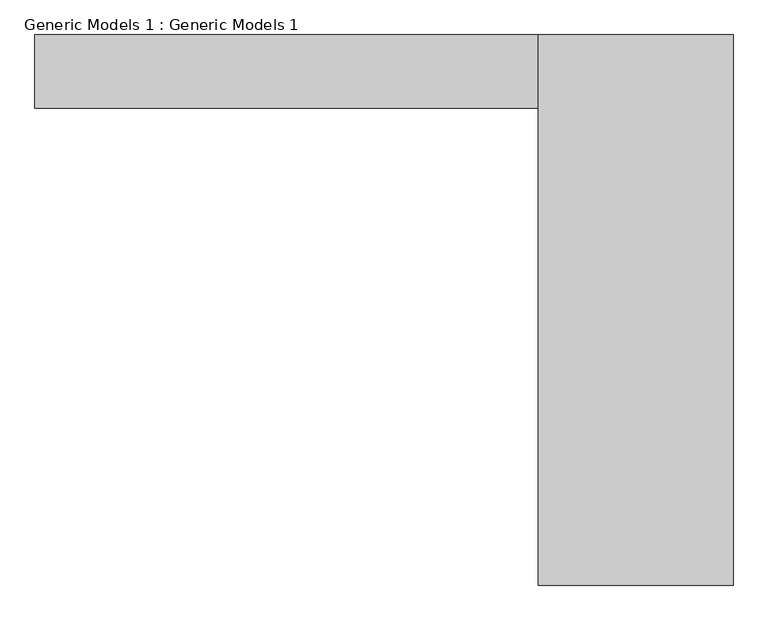
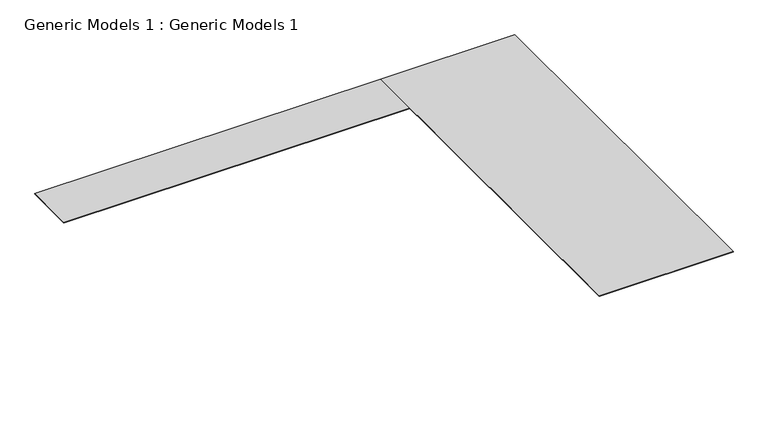
"""IFC4 building model written with IfcOpenShell, lengths in millimetres: proxy geometry, Generic Models 1 : Generic Models 1."""

from ifc_helpers import new_model, si_unit, origin, origin_with_axes, place, context, project, spatial, polyline, outline, extrude, source, transform, mapped, element, save


def generic_models_1_generic_models_1_28a2cc20(model_context):
    return source(origin(), model_context, "Body", "SweptSolid", [
        extrude(outline(polyline([(21968.4663282, 19178.0873915), (-9452.0005661, 19178.0873915), (-9452.0005661, 23749.0), (21968.4663282, 23749.0), (21968.4663282, 19178.0873915)])), origin_with_axes(), (0.0, 0.0, 1.0), 26.8572052),
        extrude(outline(polyline([(34119.235043, 23749.0), (34119.235043, -10616.9760959), (21968.4663282, -10616.9760959), (21968.4663282, 23749.0), (34119.235043, 23749.0)])), origin_with_axes(), (0.0, 0.0, 1.0), 46.7783103),
    ])


if __name__ == "__main__":
    model = new_model("IFC4")
    model_context = context("Model", 3, world=origin())
    ifc_project = project(units=[si_unit("LENGTHUNIT", "METRE", prefix="MILLI")], contexts=[model_context])
    site = spatial("IfcSite", under=ifc_project)
    building = spatial("IfcBuilding", under=site)
    placement = place(None, origin())
    generic_models_1_generic_models_1_shape = generic_models_1_generic_models_1_28a2cc20(model_context)
    element("IfcBuildingElementProxy", 1, Name="Generic Models 1 : Generic Models 1", ObjectType="Generic Models 1 : Generic Models 1", at=placement, inside=building, context=model_context, shape_type="MappedRepresentation", body=[
        mapped(generic_models_1_generic_models_1_shape, transform((0.0, 0.0, 0.0), x_axis=(1.0, 0.0, 0.0), y_axis=(0.0, 1.0, 0.0), z_axis=(0.0, 0.0, 1.0))),
    ])
    save(model, "model.ifc")
